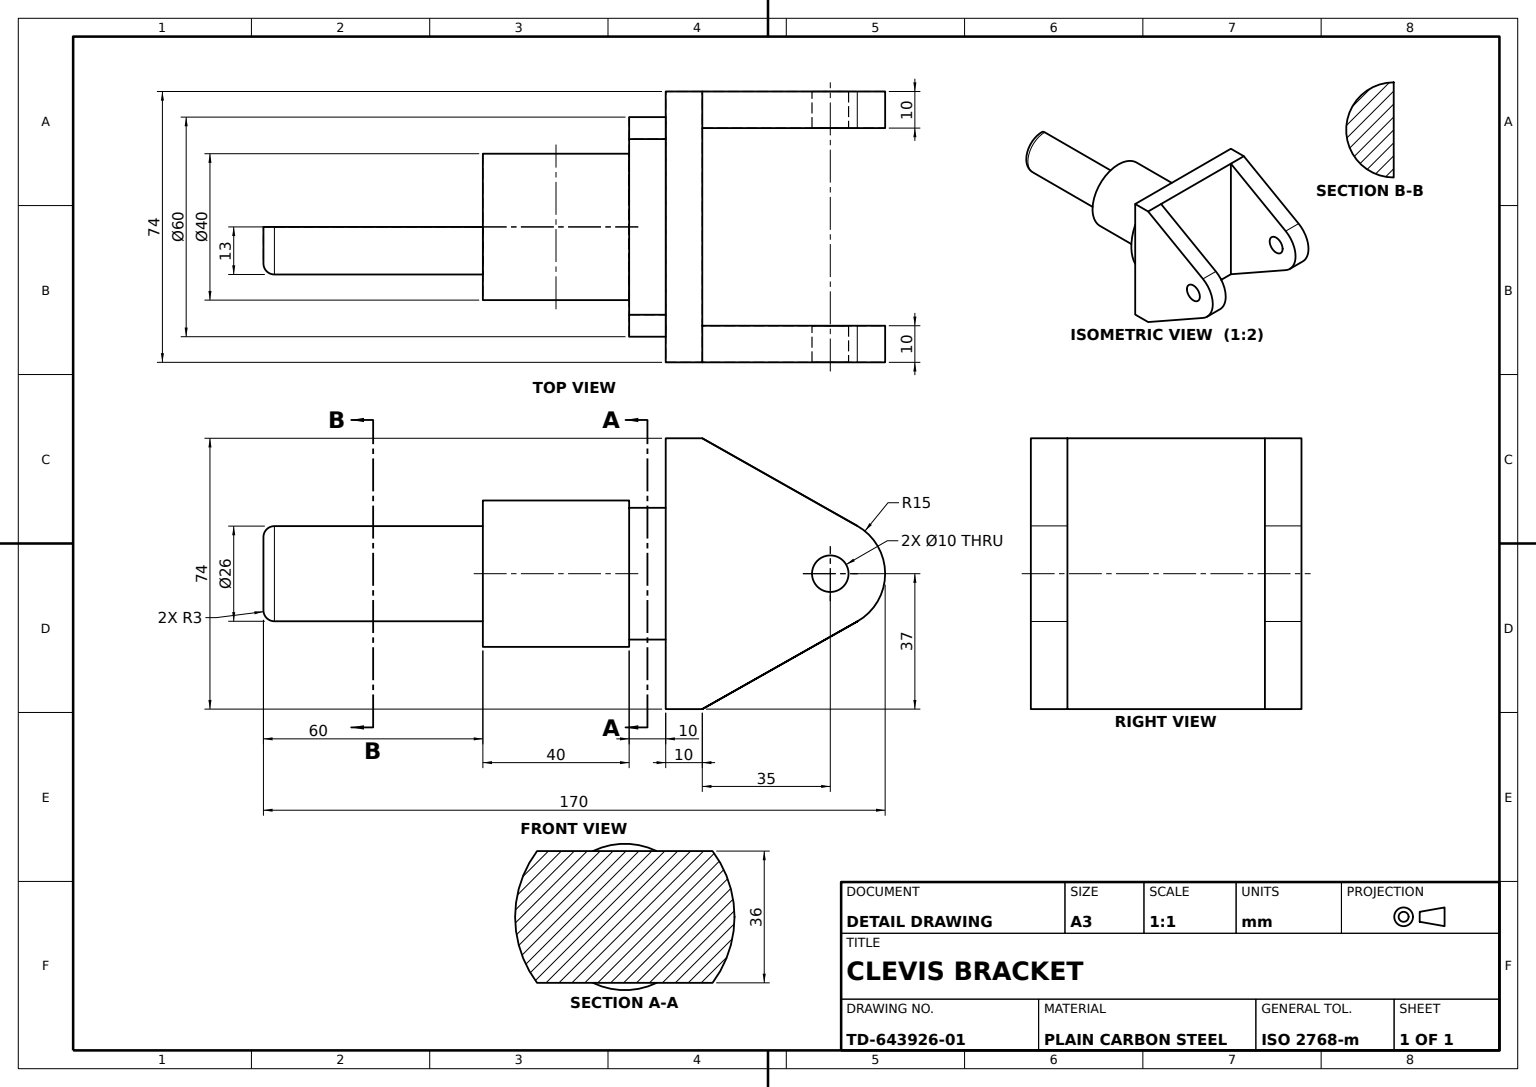
from build123d import *

# Parameters (mm, degrees)
BASE_DISC_SKETCH_60_R       = 30
BASE_DISC_60_DEPTH          = 10
BASE_START                  = -10
BASE_PROFILE_CUT_DEPTH      = 10
COLLAR_SKETCH_40_R          = 20
COLLAR_40_DEPTH             = 40
SHAFT_SKETCH_26_R           = 13
SHAFT_26_DEPTH              = 60
SHAFT_END_FILLET_R3_R       = 3
SHAFT_FLAT_CUT_DEPTH        = 30
MOUNTING_FLANGE_SKETCH_74_W = 74
MOUNTING_FLANGE_SKETCH_74_H = 74
MOUNTING_FLANGE_74_DEPTH    = 10
MOUNTING_EAR_DEPTH          = 10
EAR_HOLE_SKETCH_10_R        = 5
EAR_HOLE_10_DEPTH           = 138.640836963


with BuildPart() as part:
    # Base Disc Sketch Ø60 → Base Disc Ø60 (new body)
    with BuildSketch(Plane.XY):
        Circle(BASE_DISC_SKETCH_60_R)
    extrude(amount=BASE_DISC_60_DEPTH)

    # Base Profile Cut Sketch → Base Profile Cut (cut)
    with BuildSketch(Plane.XY.offset(10).offset(BASE_START)):
        with BuildLine():
            Line((0, 18), (-24, 18))
            ThreePointArc((-24, 18), (0, 30), (24, 18))
            Line((24, 18), (0, 18))
        make_face()
        with BuildLine():
            Line((0, -18), (24, -18))
            ThreePointArc((24, -18), (0, -30), (-24, -18))
            Line((-24, -18), (0, -18))
        make_face()
    extrude(amount=BASE_PROFILE_CUT_DEPTH, mode=Mode.SUBTRACT)

    # Collar Sketch Ø40 → Collar Ø40 (add)
    with BuildSketch(Plane.XY.offset(10)):
        with Locations(Location((0, 0, 0), (0, 0, 115.841932763))):
            Circle(COLLAR_SKETCH_40_R)
    extrude(amount=COLLAR_40_DEPTH)

    # Shaft Sketch Ø26 → Shaft Ø26 (add)
    with BuildSketch(Plane.XY.offset(50)):
        Circle(SHAFT_SKETCH_26_R)
    extrude(amount=SHAFT_26_DEPTH)

    # Shaft End Fillet R3
    shaft_end_fillet_r3_edges = [part.edges().sort_by_distance(p)[0] for p in [
        (-13, 0, 110),
    ]]
    fillet(shaft_end_fillet_r3_edges, radius=SHAFT_END_FILLET_R3_R)

    # Shaft Flat Sketch → Shaft Flat Cut (cut)
    with BuildSketch(Plane(origin=(0, 0, 0), x_dir=(0, 0, -1), z_dir=(1, 0, 0))):
        Polygon((-107, 20.022291402), (-120.828706591, 20.022291402), (-120.828706591, -20.022291402), (-107, -20.022291402), (-50, -20.022291402), (-50, 20.022291402), align=None)
    extrude(amount=-SHAFT_FLAT_CUT_DEPTH, mode=Mode.SUBTRACT)

    # Mounting Flange Sketch 74 → Mounting Flange 74 (add)
    with BuildSketch(Plane(origin=(0, 0, 0), x_dir=(-1, 0, 0), z_dir=(0, 0, -1))):
        Rectangle(MOUNTING_FLANGE_SKETCH_74_W, MOUNTING_FLANGE_SKETCH_74_H)
    extrude(amount=MOUNTING_FLANGE_74_DEPTH)

    # Mounting Ear Sketch → Mounting Ear (add)
    with BuildSketch(Plane(origin=(37, 0, 0), x_dir=(0, 0, -1), z_dir=(1, 0, 0))):
        with BuildLine():
            Line((10, 37), (52.377859531, 13.060137394))
            ThreePointArc((52.377859531, 13.060137394), (60, 0), (52.377859531, -13.060137394))
            Line((52.377859531, -13.060137394), (10, -37))
            Line((10, -37), (10, 37))
        make_face()
    mounting_ear = extrude(amount=-MOUNTING_EAR_DEPTH)

    # Mounting Ear Mirror: Mounting Ear across plane
    add(mounting_ear.mirror(Plane(origin=(0, 0, 0), x_dir=(0, 0, 1), z_dir=(1, 0, 0))))

    # Ear Hole Sketch Ø10 → Ear Hole Ø10 (cut, through all)
    with BuildSketch(Plane(origin=(37, 0, 0), x_dir=(0, 0, -1), z_dir=(1, 0, 0))):
        with Locations((45, 0)):
            Circle(EAR_HOLE_SKETCH_10_R)
    extrude(amount=-EAR_HOLE_10_DEPTH, mode=Mode.SUBTRACT)


solid = part.part
